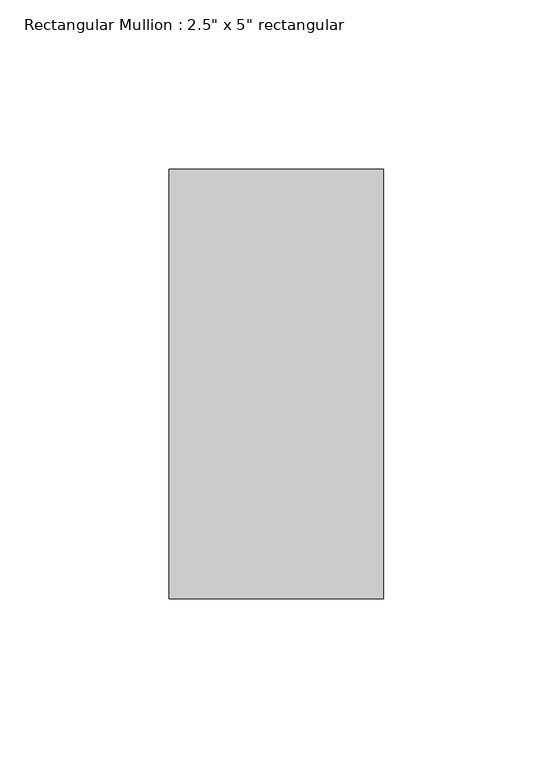
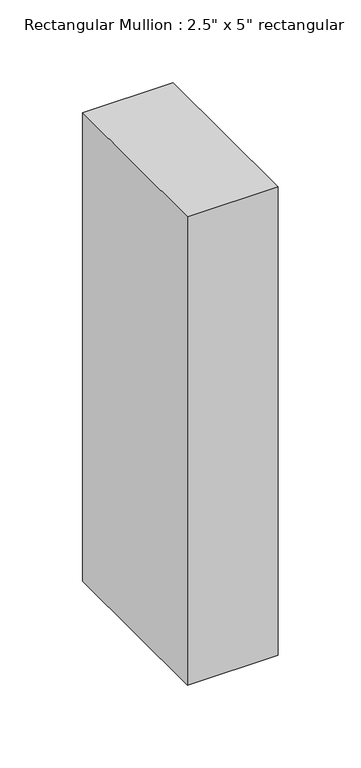
"""IFC4 building model written with IfcOpenShell, lengths in millimetres: member geometry."""

from ifc_helpers import new_model, si_unit, frame, origin, place, context, project, spatial, polyline, outline, extrude, source, transform, mapped, element, save


def member_9f7b9c5b(model_context):
    return source(origin(), model_context, "Body", "SweptSolid", [
        extrude(outline(polyline([(0.0, 63.5), (0.0, -63.5), (-63.5, -63.5), (-63.5, 63.5), (0.0, 63.5)])), frame((0.0, 0.0, -346.075), z_axis=(0.0, 0.0, 1.0), x_axis=(1.0, 0.0, 0.0)), (0.0, 0.0, 1.0), 346.075),
    ])


if __name__ == "__main__":
    model = new_model("IFC4")
    model_context = context("Model", 3, world=origin())
    ifc_project = project(units=[si_unit("LENGTHUNIT", "METRE", prefix="MILLI")], contexts=[model_context])
    site = spatial("IfcSite", under=ifc_project)
    building = spatial("IfcBuilding", under=site)
    placement = place(None, origin())
    member_shape = member_9f7b9c5b(model_context)
    element("IfcMember", 1, ObjectType="Rectangular Mullion : 2.5\" x 5\" rectangular", at=placement, inside=building, context=model_context, shape_type="MappedRepresentation", body=[
        mapped(member_shape, transform((0.0, 0.0, 0.0), x_axis=(1.0, 0.0, 0.0), y_axis=(0.0, 1.0, 0.0), z_axis=(0.0, 0.0, 1.0))),
    ])
    save(model, "model.ifc")

# Revit data of these elements
# Type "Rectangular Mullion : 2.5\" x 5\" rectangular"
#   built-in parameter 1007304 = 0.416667 (stored number, unit not read)
#   built-in parameter 1007301 = 0.104167 (stored number, unit not read)
#   built-in parameter 1007300 = 0.104167 (stored number, unit not read)
# Element 1 (IfcMember, "Rectangular Mullion : 2.5\" x 5\" rectangular")
#   Materials on its faces: "Aluminum"
# Materials
#   "Aluminum": class "Metal", colour RGB 247 247 247, transparency 0, Description = "Aluminum 6061", Cost = 0
